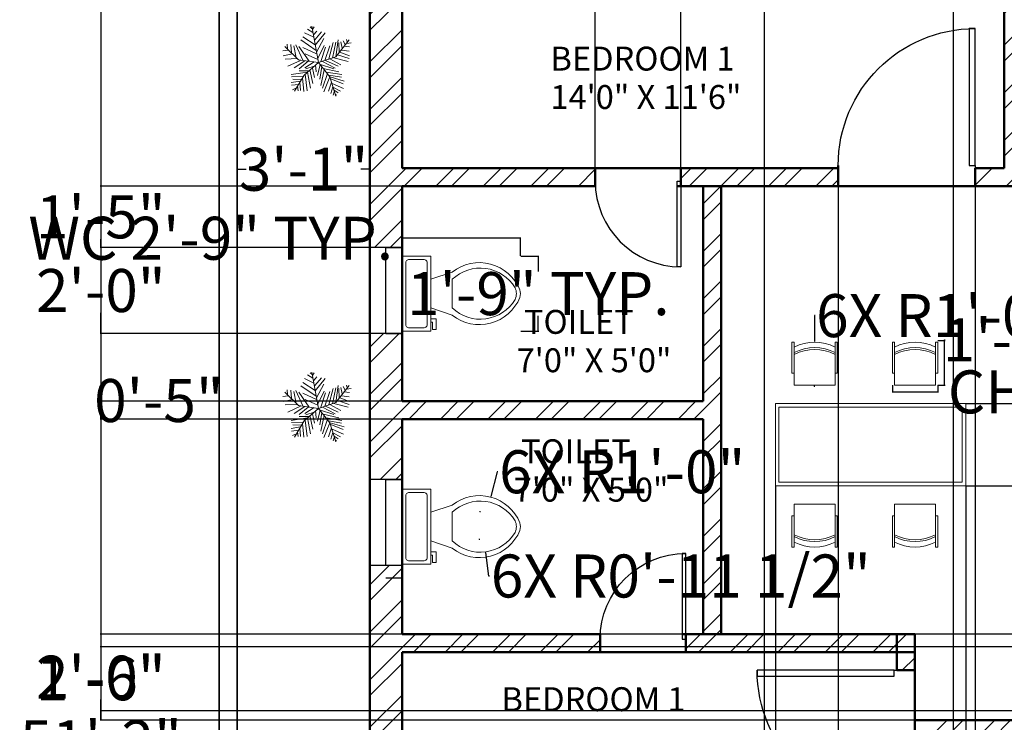
# Model space of a CAD drawing. Units: inches. Extents: x -40 to 578, y -482 to 237.
# Tile 4 of 7: x -26 to 249, y -129 to 67. Entities that reach past the tile are written whole.
import ezdxf

# ---------------------------------------------------------------- set-up
doc = ezdxf.new("R2010")
doc.units = ezdxf.units.IN
doc.header["$MEASUREMENT"] = 0
for name, color, linetype, lineweight in [('A-ANNO-DIMS', 2, 'Continuous', 18), ('A-AREA-IDEN', 240, 'Continuous', 25), ('A-FLOR-FIXT', 4, 'Continuous', 18), ('A-FURN', 4, 'Continuous', 18), ('A-WALL-PATT', 252, 'Continuous', 13), ('C-PROP', 3, 'Continuous', 35), ('DOORS', 2, 'Continuous', 25), ('L-PLNT', 94, 'Continuous', 13), ('WALLS', 3, 'Continuous', 50), ('WINDOWS', 241, 'Continuous', 25)]:
    doc.layers.add(name, color=color, linetype=linetype, lineweight=lineweight)
doc.styles.get("Standard").update_dxf_attribs({"font": 'arial.ttf'})
doc.dimstyles.get("Standard").update_dxf_attribs({"dimtxt": 12, "dimasz": 0.18, "dimexe": 0.18, "dimexo": 0.0625, "dimgap": 0.09, "dimtad": 0, "dimtih": 1, "dimtoh": 1, "dimdec": 0, "dimzin": 0, "dimdsep": 46, "dimlunit": 3, "dimtxsty": 'Standard', "dimcen": 0.09, "dimadec": 0, "dimazin": 0, "dimtfac": 1, "dimtdec": 0, "dimtofl": 0, "dimtmove": 0, "dimatfit": 3, "dimfxl": 1, "dimtolj": 1, "dimtzin": 0, "dimarcsym": 0})

# ---------------------------------------------------------------- blocks, each defined once
blk = doc.blocks.new('Toilet - top')
for p, q in [((9.5, -6), (9.5, -2)), ((-8, -8.5), (-8, -8)), ((-7, -8), (-7, -9.5)), ((-4, -8), (-6, -14)), ((4, -8), (6, -14)), ((-10, -8.5), (-8, -8.5)), ((-10, -9.5), (-10, -8.5)), ((-7, -9.5), (-10, -9.5)), ((4, -14), (-4, -14))]:
    blk.add_line(p, q)
blk.add_lwpolyline([(10.5, -8), (10.5, 0), (-10.5, 0), (-10.5, -8)], close=True)
for points in [[(-9.5, -2), (-9.5, -6)], [(8.5, -1), (-8.5, -1)], [(-8.5, -7), (8.5, -7)]]:
    blk.add_lwpolyline(points)
for centre, radius, start, end in [((-8.62, -1.88), 0.884, 81.8699, 188.1301), ((8.62, -1.88), 0.884, 351.8699, 98.1301), ((-8.62, -6.12), 0.884, 171.8699, 278.1301), ((8.62, -6.12), 0.884, 261.8699, 8.1301), ((3.52, -21.58), 12.17, 141.4691, 247.9714), ((4.2, -21.82), 11.33, 136.3677, 238.9468), ((-3.52, -21.58), 12.17, 292.0284, 38.5307), ((-4.2, -21.82), 11.33, 301.053, 43.6321), ((0, -27.88), 4, 245.7318, 294.2682), ((0, -29), 4, 254.8605, 285.1395)]:
    blk.add_arc(centre, radius, start, end)
blk = doc.blocks.new('*U10')
for p, q in [((0, 0), (0, -6)), ((40, 0), (40, -6))]:
    blk.add_line(p, q)
blk.add_lwpolyline([(0, 0), (0, 40), (1.75, 40), (1.75, 0)], close=True)
blk.add_arc((0, 0), 40, 0, 90)
blk = doc.blocks.new('*U14')
for p, q in [((-185.1152, 1008.5578), (-553.1612, 1185.4942)), ((-221.9198, 1197.3052), (-433.5526, 1338.8594)), ((-258.7244, 1362.456), (-332.3336, 1421.4348)), ((0, 0), (-266.7, 1447.8)), ((-231.1146, 1315.2628), (-166.7002, 1421.4348)), ((-194.31, 1102.9442), (-65.4812, 1256.284)), ((-148.3106, 914.1968), (118.5418, 1220.9018)), ((-129.8956, 701.8528), (265.7602, 1185.4942)), ((-93.091, 489.5342), (-700.3796, 902.3858)), ((-129.8956, 713.6638), (-626.7704, 1032.1544)), ((-74.7014, 418.7444), (219.7608, 961.39)), ((412.9786, 147.447), (587.8068, 796.2392)), ((560.197, 182.8292), (698.2206, 819.8358)), ((685.8, 228.6), (1219.2, 914.4)), ((689.0258, 230.0224), (790.2448, 914.1968)), ((891.4384, 831.6214), (946.658, 572.1096)), ((983.4626, 867.0036), (1066.2666, 725.4494)), ((1121.4862, 925.9824), (1149.0706, 831.6214)), ((-1206.4492, 501.3198), (-1418.082, 465.9376)), ((-800.1, 114.3), (-1333.5, 647.7)), ((-1234.059, 536.7274), (-1252.4486, 737.2604)), ((-1105.2302, 725.4494), (-1077.6458, 395.1732)), ((-976.4268, 666.4706), (-884.4026, 194.6402)), ((-902.8176, 713.6638), (-617.5756, 100.2538)), ((-369.1382, 53.086), (-783.1836, 642.874)), ((-617.5756, 607.4918), (-74.7014, 347.98)), ((-28.6766, 171.0436), (228.9556, 678.2816)), ((100.1268, 41.275), (284.1498, 619.2774)), ((256.5654, 88.4682), (449.7832, 666.4706)), ((808.6344, 784.4282), (827.0494, 418.7444)), ((845.439, 418.7444), (1241.0948, 277.1902)), ((919.0482, 501.3198), (1222.6798, 454.152)), ((1029.462, 654.685), (1241.0948, 631.0884)), ((1112.2914, 760.8316), (1296.3144, 784.4282)), ((-1031.621, 347.98), (-1399.667, 277.1902)), ((-847.598, 159.2326), (-1326.0578, 135.636)), ((-718.7946, 88.4682), (-1215.644, -147.447)), ((-543.9664, 76.6572), (-967.2066, -206.4512)), ((0, 0), (-800.1, 114.3)), ((-405.9428, 53.086), (-764.794, -241.8334)), ((0, 0), (-571.5, -495.3)), ((-166.7002, 29.4894), (-543.9664, -206.4512)), ((-525.5514, 347.98), (-28.6766, 123.8504)), ((0, 0), (685.8, 228.6)), ((0, 0), (457.2, -571.5)), ((164.5412, 41.275), (661.416, -218.2368)), ((284.1498, 88.4682), (781.0246, -147.447)), ((458.978, 147.447), (891.4384, -88.4682)), ((615.4166, 194.6402), (1185.8752, 41.275)), ((753.4148, 312.5978), (1222.6798, 159.2326)), ((-442.7474, -383.3876), (-1086.8406, -477.7486)), ((-387.5278, -324.4088), (-764.794, -324.4088)), ((-166.7002, -147.447), (-507.1618, -253.619)), ((-433.5526, -383.3876), (-323.1134, -1020.3688)), ((-341.5284, -289.0012), (-221.9198, -831.6214)), ((-240.3094, -218.2368), (-157.5054, -595.7062)), ((-120.7008, -88.4682), (-93.091, -371.5766)), ((63.3222, -76.6826), (-37.8714, -513.1308)), ((44.9326, -64.897), (615.4166, -241.8334)), ((127.7366, -159.258), (54.1274, -654.685)), ((228.9556, -289.0012), (90.932, -914.1968)), ((192.151, -230.0224), (817.8292, -371.5766)), ((311.7596, -383.3876), (937.4378, -477.7486)), ((-718.7946, -737.2604), (-1086.8406, -796.2392)), ((-617.5756, -548.5384), (-1077.6458, -560.324)), ((-681.9646, -666.496), (-1022.4262, -654.685)), ((-571.5, -495.3), (-952.5, -1143)), ((-737.1842, -784.4536), (-709.5744, -1114.7298)), ((-635.9652, -607.5172), (-580.771, -1150.1374)), ((-525.5514, -465.963), (-451.9422, -1126.5408)), ((357.759, -430.5554), (164.5412, -1020.3688)), ((458.978, -572.1096), (210.5406, -1161.923)), ((514.1976, -772.6426), (403.7838, -1138.3264)), ((412.9786, -501.3452), (919.0482, -583.9206)), ((457.2, -571.5), (685.8, -1333.5)), ((468.1982, -572.1096), (1029.462, -737.2604)), ((486.5878, -642.8994), (983.4626, -843.4324)), ((-783.1836, -867.029), (-1077.6458, -902.4112)), ((-875.2078, -1008.5832), (-1040.8412, -1079.3476)), ((-829.2084, -937.7934), (-810.7934, -1126.5408)), ((578.612, -961.39), (495.7826, -1232.7128)), ((541.8074, -831.6214), (992.6574, -1032.1544)), ((578.612, -973.1756), (873.0488, -1138.3264)), ((624.6114, -1161.923), (587.8068, -1291.6916)), ((624.6114, -1102.9442), (781.0246, -1209.1162)), ((679.8056, -1268.095), (716.6102, -1291.6916))]:
    blk.add_line(p, q)
blk = doc.blocks.new('*D20')
at = {"layer": 'A-ANNO-DIMS', "color": 0, "lineweight": -2, "transparency": 16777216}
for p, q in [((34.74, 26.4), (34.74, 24.97)), ((34.92, 25.15), (37.2, 25.15)), ((71.56, 25.15), (69.27, 25.15)), ((71.74, 26.4), (71.74, 24.97))]:
    blk.add_line(p, q, dxfattribs=at)
at = {"layer": 'A-ANNO-DIMS', "color": 0, "transparency": 16777216}
for points in [[(34.92, 25.18), (34.92, 25.12), (34.74, 25.15)], [(71.56, 25.18), (71.56, 25.12), (71.74, 25.15)]]:
    blk.add_solid(points, dxfattribs=at)
at = {"layer": 'Defpoints', "color": 0, "transparency": 16777216}
for p in [(34.74, 26.46), (34.74, 25.15), (71.74, 26.46)]:
    blk.add_point(p, dxfattribs=at)
at = {"layer": 'A-ANNO-DIMS', "color": 0, "transparency": 16777216, "insert": (53.24, 25.15), "char_height": 12, "attachment_point": 5}
blk.add_mtext('\\A1;3\'-1"', dxfattribs=at)
blk = doc.blocks.new('CHAIR-DINING')
for p, q in [((0.63, 0), (0.63, 10.59)), ((12.01, 10.59), (12.01, 0)), ((12.01, 0), (0.63, 0))]:
    blk.add_line(p, q)
for points in [[(0.63, 11.98), (0, 11.98), (0, 3.3), (0.63, 3.3)], [(12.64, 11.98), (12.01, 11.98), (12.01, 3.3), (12.64, 3.3)]]:
    blk.add_lwpolyline(points, close=True)
for centre in [(6.32, -0.34), (6.32, -1.87), (6.32, -2.38)]:
    blk.add_arc(centre, 12.32, 62.4906, 117.5094)
blk = doc.blocks.new('*D30')
at = {"layer": 'A-ANNO-DIMS', "color": 0, "lineweight": -2, "transparency": 16777216}
for p, q in [((217.52, -35.11), (217.52, -37.13)), ((230.16, -35.11), (230.16, -37.13)), ((217.7, -36.95), (229.98, -36.95)), ((230.16, -36.95), (230.34, -36.95))]:
    blk.add_line(p, q, dxfattribs=at)
at = {"layer": 'A-ANNO-DIMS', "color": 0, "transparency": 16777216}
for points in [[(217.7, -36.92), (217.7, -36.98), (217.52, -36.95)], [(229.98, -36.92), (229.98, -36.98), (230.16, -36.95)]]:
    blk.add_solid(points, dxfattribs=at)
at = {"layer": 'Defpoints', "color": 0, "transparency": 16777216}
for p in [(217.52, -35.05), (230.16, -35.05), (230.16, -36.95)]:
    blk.add_point(p, dxfattribs=at)
at = {"layer": 'A-ANNO-DIMS', "color": 0, "transparency": 16777216, "insert": (309.32, -36.95), "char_height": 12, "attachment_point": 5}
blk.add_mtext('\\A1;CHAIR 1\'-0 1/2" TYP.', dxfattribs=at)
blk = doc.blocks.new('*D31')
at = {"layer": 'A-ANNO-DIMS', "color": 0, "lineweight": -2, "transparency": 16777216}
for p, q in [((230.22, -22.61), (232.23, -22.61)), ((232.05, -22.61), (232.05, -22.43)), ((232.05, -22.43), (232.23, -22.43)), ((232.05, -34.87), (232.05, -22.79)), ((230.22, -35.05), (232.23, -35.05))]:
    blk.add_line(p, q, dxfattribs=at)
at = {"layer": 'A-ANNO-DIMS', "color": 0, "transparency": 16777216}
for points in [[(232.02, -22.79), (232.08, -22.79), (232.05, -22.61)], [(232.02, -34.87), (232.08, -34.87), (232.05, -35.05)]]:
    blk.add_solid(points, dxfattribs=at)
at = {"layer": 'Defpoints', "color": 0, "transparency": 16777216}
for p in [(230.16, -22.61), (232.05, -22.61), (230.16, -35.05)]:
    blk.add_point(p, dxfattribs=at)
at = {"layer": 'A-ANNO-DIMS', "color": 0, "transparency": 16777216, "insert": (282.31, -22.43), "char_height": 12, "attachment_point": 5}
blk.add_mtext('\\A1;1\'-0 1/2" TYP.', dxfattribs=at)
blk = doc.blocks.new('*D34')
at = {"layer": 'A-ANNO-DIMS', "color": 0, "lineweight": -2, "transparency": 16777216}
for p, q in [((80.74, 5.9), (80.56, 5.9)), ((80.74, 1.01), (80.74, 6.08)), ((113.6, 5.9), (80.92, 5.9)), ((113.78, 1.01), (113.78, 6.08))]:
    blk.add_line(p, q, dxfattribs=at)
at = {"layer": 'A-ANNO-DIMS', "color": 0, "transparency": 16777216}
for points in [[(80.92, 5.93), (80.92, 5.87), (80.74, 5.9)], [(113.6, 5.93), (113.6, 5.87), (113.78, 5.9)]]:
    blk.add_solid(points, dxfattribs=at)
at = {"layer": 'Defpoints', "color": 0, "transparency": 16777216}
for p in [(80.74, 5.9), (80.74, 0.95), (113.78, 0.95)]:
    blk.add_point(p, dxfattribs=at)
at = {"layer": 'A-ANNO-DIMS', "color": 0, "transparency": 16777216, "insert": (27.36, 5.9), "char_height": 12, "attachment_point": 5}
blk.add_mtext('\\A1;WC 2\'-9" TYP.', dxfattribs=at)
blk = doc.blocks.new('*D35')
at = {"layer": 'A-ANNO-DIMS', "color": 0, "lineweight": -2, "transparency": 16777216}
for p, q in [((113.85, 0.95), (118.92, 0.95)), ((118.74, 0.77), (118.74, -3.34)), ((118.74, -19.87), (118.74, -15.77)), ((113.85, -20.05), (118.92, -20.05))]:
    blk.add_line(p, q, dxfattribs=at)
at = {"layer": 'A-ANNO-DIMS', "color": 0, "transparency": 16777216}
for points in [[(118.71, 0.77), (118.77, 0.77), (118.74, 0.95)], [(118.71, -19.87), (118.77, -19.87), (118.74, -20.05)]]:
    blk.add_solid(points, dxfattribs=at)
at = {"layer": 'Defpoints', "color": 0, "transparency": 16777216}
for p in [(113.78, 0.95), (118.74, 0.95), (113.78, -20.05)]:
    blk.add_point(p, dxfattribs=at)
at = {"layer": 'A-ANNO-DIMS', "color": 0, "transparency": 16777216, "insert": (118.74, -9.55), "char_height": 12, "attachment_point": 5}
blk.add_mtext('\\A1;1\'-9" TYP.', dxfattribs=at)
blk = doc.blocks.new('*D42')
at = {"layer": 'A-ANNO-DIMS', "color": 0, "lineweight": -2, "transparency": 16777216}
for p, q in [((71.78, -441.49), (71.78, 219.12)), ((71.96, 218.94), (110.77, 218.94)), ((181.65, 218.94), (142.84, 218.94)), ((181.83, -441.49), (181.83, 219.12))]:
    blk.add_line(p, q, dxfattribs=at)
at = {"layer": 'A-ANNO-DIMS', "color": 0, "transparency": 16777216}
for points in [[(71.96, 218.97), (71.96, 218.91), (71.78, 218.94)], [(181.65, 218.97), (181.65, 218.91), (181.83, 218.94)]]:
    blk.add_solid(points, dxfattribs=at)
at = {"layer": 'Defpoints', "color": 0, "transparency": 16777216}
for p in [(181.83, 218.94), (71.78, -441.55), (181.83, -441.55)]:
    blk.add_point(p, dxfattribs=at)
at = {"layer": 'A-ANNO-DIMS', "color": 0, "transparency": 16777216, "insert": (126.81, 218.94), "char_height": 12, "attachment_point": 5}
blk.add_mtext('\\A1;9\'-2"', dxfattribs=at)
blk = doc.blocks.new('*D44')
at = {"layer": 'A-ANNO-DIMS', "color": 0, "lineweight": -2, "transparency": 16777216}
for p, q in [((29.68, 172.45), (-3.49, 172.45)), ((-3.31, 172.27), (-3.31, -128.34)), ((-3.31, -441.37), (-3.31, -140.77)), ((29.68, -441.55), (-3.49, -441.55))]:
    blk.add_line(p, q, dxfattribs=at)
at = {"layer": 'A-ANNO-DIMS', "color": 0, "transparency": 16777216}
for points in [[(-3.34, 172.27), (-3.28, 172.27), (-3.31, 172.45)], [(-3.34, -441.37), (-3.28, -441.37), (-3.31, -441.55)]]:
    blk.add_solid(points, dxfattribs=at)
at = {"layer": 'Defpoints', "color": 0, "transparency": 16777216}
for p in [(-3.31, 172.45), (29.74, 172.45), (29.74, -441.55)]:
    blk.add_point(p, dxfattribs=at)
at = {"layer": 'A-ANNO-DIMS', "color": 0, "transparency": 16777216, "insert": (-3.31, -134.55), "char_height": 12, "attachment_point": 5}
blk.add_mtext('\\A1;51\'-2"', dxfattribs=at)
blk = doc.blocks.new('*D52')
at = {"layer": 'A-ANNO-DIMS', "color": 0, "lineweight": -2, "transparency": 16777216}
for p, q in [((234.57, -377.49), (234.57, 219.12)), ((234.75, 218.94), (265.48, 218.94)), ((265.66, -377.49), (265.66, 219.12)), ((265.66, 218.94), (265.84, 218.94))]:
    blk.add_line(p, q, dxfattribs=at)
at = {"layer": 'A-ANNO-DIMS', "color": 0, "transparency": 16777216}
for points in [[(234.75, 218.97), (234.75, 218.91), (234.57, 218.94)], [(265.48, 218.97), (265.48, 218.91), (265.66, 218.94)]]:
    blk.add_solid(points, dxfattribs=at)
at = {"layer": 'Defpoints', "color": 0, "transparency": 16777216}
for p in [(265.66, 218.94), (234.57, -377.55), (265.66, -377.55)]:
    blk.add_point(p, dxfattribs=at)
at = {"layer": 'A-ANNO-DIMS', "color": 0, "transparency": 16777216, "insert": (281.98, 218.94), "char_height": 12, "attachment_point": 5}
blk.add_mtext('\\A1;2\'-7"', dxfattribs=at)
blk = doc.blocks.new('*D54')
at = {"layer": 'A-ANNO-DIMS', "color": 0, "lineweight": -2, "transparency": 16777216}
for p, q in [((202.4, 25.39), (202.4, -474.78)), ((240.62, 25.39), (240.62, -474.78)), ((202.58, -474.6), (205.48, -474.6)), ((240.44, -474.6), (237.55, -474.6))]:
    blk.add_line(p, q, dxfattribs=at)
at = {"layer": 'A-ANNO-DIMS', "color": 0, "transparency": 16777216}
for points in [[(202.58, -474.57), (202.58, -474.63), (202.4, -474.6)], [(240.44, -474.57), (240.44, -474.63), (240.62, -474.6)]]:
    blk.add_solid(points, dxfattribs=at)
at = {"layer": 'Defpoints', "color": 0, "transparency": 16777216}
for p in [(202.4, 25.45), (240.62, 25.45), (240.62, -474.6)]:
    blk.add_point(p, dxfattribs=at)
at = {"layer": 'A-ANNO-DIMS', "color": 0, "transparency": 16777216, "insert": (221.51, -474.6), "char_height": 12, "attachment_point": 5}
blk.add_mtext('\\A1;3\'-2"', dxfattribs=at)
blk = doc.blocks.new('*D55')
at = {"layer": 'A-ANNO-DIMS', "color": 0, "lineweight": -2, "transparency": 16777216}
for p, q in [((134.6, 25.51), (134.6, 219.12)), ((134.78, 218.94), (158.35, 218.94)), ((158.53, 25.51), (158.53, 219.12)), ((158.53, 218.94), (158.71, 218.94))]:
    blk.add_line(p, q, dxfattribs=at)
at = {"layer": 'A-ANNO-DIMS', "color": 0, "transparency": 16777216}
for points in [[(134.78, 218.97), (134.78, 218.91), (134.6, 218.94)], [(158.35, 218.97), (158.35, 218.91), (158.53, 218.94)]]:
    blk.add_solid(points, dxfattribs=at)
at = {"layer": 'Defpoints', "color": 0, "transparency": 16777216}
for p in [(158.53, 218.94), (134.6, 25.45), (158.53, 25.45)]:
    blk.add_point(p, dxfattribs=at)
at = {"layer": 'A-ANNO-DIMS', "color": 0, "transparency": 16777216, "insert": (174.86, 218.94), "char_height": 12, "attachment_point": 5}
blk.add_mtext('\\A1;2\'-0"', dxfattribs=at)
blk = doc.blocks.new('*D56')
at = {"layer": 'A-ANNO-DIMS', "color": 0, "lineweight": -2, "transparency": 16777216}
for p, q in [((71.68, 3.32), (-3.49, 3.32)), ((-3.31, 3.14), (-3.31, -2.46)), ((-3.31, -20.5), (-3.31, -14.9)), ((71.68, -20.68), (-3.49, -20.68))]:
    blk.add_line(p, q, dxfattribs=at)
at = {"layer": 'A-ANNO-DIMS', "color": 0, "transparency": 16777216}
for points in [[(-3.34, 3.14), (-3.28, 3.14), (-3.31, 3.32)], [(-3.34, -20.5), (-3.28, -20.5), (-3.31, -20.68)]]:
    blk.add_solid(points, dxfattribs=at)
at = {"layer": 'Defpoints', "color": 0, "transparency": 16777216}
for p in [(-3.31, 3.32), (71.74, 3.32), (71.74, -20.68)]:
    blk.add_point(p, dxfattribs=at)
at = {"layer": 'A-ANNO-DIMS', "color": 0, "transparency": 16777216, "insert": (-3.31, -8.68), "char_height": 12, "attachment_point": 5}
blk.add_mtext('\\A1;2\'-0"', dxfattribs=at)
blk = doc.blocks.new('*D57')
at = {"layer": 'A-ANNO-DIMS', "color": 0, "lineweight": -2, "transparency": 16777216}
for p, q in [((164.68, -39.55), (-3.49, -39.55)), ((-3.31, -39.55), (-3.31, -39.37)), ((-3.31, -39.37), (-3.13, -39.37)), ((-3.31, -44.37), (-3.31, -39.73)), ((164.68, -44.55), (-3.49, -44.55))]:
    blk.add_line(p, q, dxfattribs=at)
at = {"layer": 'A-ANNO-DIMS', "color": 0, "transparency": 16777216}
for points in [[(-3.34, -39.73), (-3.28, -39.73), (-3.31, -39.55)], [(-3.34, -44.37), (-3.28, -44.37), (-3.31, -44.55)]]:
    blk.add_solid(points, dxfattribs=at)
at = {"layer": 'Defpoints', "color": 0, "transparency": 16777216}
for p in [(-3.31, -39.55), (164.74, -39.55), (164.74, -44.55)]:
    blk.add_point(p, dxfattribs=at)
at = {"layer": 'A-ANNO-DIMS', "color": 0, "transparency": 16777216, "insert": (12.91, -39.37), "char_height": 12, "attachment_point": 5}
blk.add_mtext('\\A1;0\'-5"', dxfattribs=at)
blk = doc.blocks.new('*D58')
at = {"layer": 'A-ANNO-DIMS', "color": 0, "lineweight": -2, "transparency": 16777216}
for p, q in [((80.68, 20.45), (-3.49, 20.45)), ((-3.31, 20.27), (-3.31, 18.1)), ((-3.31, 3.5), (-3.31, 5.67)), ((80.68, 3.32), (-3.49, 3.32))]:
    blk.add_line(p, q, dxfattribs=at)
at = {"layer": 'A-ANNO-DIMS', "color": 0, "transparency": 16777216}
for points in [[(-3.34, 20.27), (-3.28, 20.27), (-3.31, 20.45)], [(-3.34, 3.5), (-3.28, 3.5), (-3.31, 3.32)]]:
    blk.add_solid(points, dxfattribs=at)
at = {"layer": 'Defpoints', "color": 0, "transparency": 16777216}
for p in [(-3.31, 20.45), (80.74, 20.45), (80.74, 3.32)]:
    blk.add_point(p, dxfattribs=at)
at = {"layer": 'A-ANNO-DIMS', "color": 0, "transparency": 16777216, "insert": (-3.31, 11.88), "char_height": 12, "attachment_point": 5}
blk.add_mtext('\\A1;1\'-5"', dxfattribs=at)
blk = doc.blocks.new('*D66')
at = {"layer": 'A-ANNO-DIMS', "color": 0, "lineweight": -2, "transparency": 16777216}
for p, q in [((289.5, -104.55), (-3.49, -104.55)), ((-3.31, -104.73), (-3.31, -110.34)), ((-3.31, -128.37), (-3.31, -122.77)), ((289.5, -128.55), (-3.49, -128.55))]:
    blk.add_line(p, q, dxfattribs=at)
at = {"layer": 'A-ANNO-DIMS', "color": 0, "transparency": 16777216}
for points in [[(-3.34, -104.73), (-3.28, -104.73), (-3.31, -104.55)], [(-3.34, -128.37), (-3.28, -128.37), (-3.31, -128.55)]]:
    blk.add_solid(points, dxfattribs=at)
at = {"layer": 'Defpoints', "color": 0, "transparency": 16777216}
for p in [(289.56, -104.55), (-3.31, -128.55), (289.56, -128.55)]:
    blk.add_point(p, dxfattribs=at)
at = {"layer": 'A-ANNO-DIMS', "color": 0, "transparency": 16777216, "insert": (-3.31, -116.55), "char_height": 12, "attachment_point": 5}
blk.add_mtext('\\A1;2\'-0"', dxfattribs=at)
blk = doc.blocks.new('*D68')
at = {"layer": 'A-ANNO-DIMS', "color": 0, "lineweight": -2, "transparency": 16777216}
for p, q in [((321.44, -108.06), (-3.49, -108.06)), ((-3.31, -108.24), (-3.31, -110.78)), ((-3.31, -125.74), (-3.31, -123.21)), ((321.44, -125.92), (-3.49, -125.92))]:
    blk.add_line(p, q, dxfattribs=at)
at = {"layer": 'A-ANNO-DIMS', "color": 0, "transparency": 16777216}
for points in [[(-3.34, -108.24), (-3.28, -108.24), (-3.31, -108.06)], [(-3.34, -125.74), (-3.28, -125.74), (-3.31, -125.92)]]:
    blk.add_solid(points, dxfattribs=at)
at = {"layer": 'Defpoints', "color": 0, "transparency": 16777216}
for p in [(321.5, -108.06), (-3.31, -125.92), (321.5, -125.92)]:
    blk.add_point(p, dxfattribs=at)
at = {"layer": 'A-ANNO-DIMS', "color": 0, "transparency": 16777216, "insert": (-3.31, -116.99), "char_height": 12, "attachment_point": 5}
blk.add_mtext('\\A1;1\'-6"', dxfattribs=at)
blk = doc.blocks.new('*D71')
at = {"layer": 'A-ANNO-DIMS', "color": 0, "lineweight": -2, "transparency": 16777216}
for p, q in [((184.88, -63.19), (184.88, -474.78)), ((237.97, -63.19), (237.97, -474.78)), ((185.06, -474.6), (195.15, -474.6)), ((237.79, -474.6), (227.71, -474.6))]:
    blk.add_line(p, q, dxfattribs=at)
at = {"layer": 'A-ANNO-DIMS', "color": 0, "transparency": 16777216}
for points in [[(185.06, -474.57), (185.06, -474.63), (184.88, -474.6)], [(237.79, -474.57), (237.79, -474.63), (237.97, -474.6)]]:
    blk.add_solid(points, dxfattribs=at)
at = {"layer": 'Defpoints', "color": 0, "transparency": 16777216}
for p in [(184.88, -63.12), (237.97, -63.12), (237.97, -474.6)]:
    blk.add_point(p, dxfattribs=at)
at = {"layer": 'A-ANNO-DIMS', "color": 0, "transparency": 16777216, "insert": (211.43, -474.6), "char_height": 12, "attachment_point": 5}
blk.add_mtext('\\A1;4\'-5"', dxfattribs=at)
blk = doc.blocks.new('*D72')
at = {"layer": 'A-ANNO-DIMS', "color": 0, "lineweight": -2, "transparency": 16777216}
for p, q in [((238.04, -40.21), (516.97, -40.21)), ((516.79, -40.39), (516.79, -45.55)), ((516.79, -62.94), (516.79, -57.78)), ((238.04, -63.12), (516.97, -63.12))]:
    blk.add_line(p, q, dxfattribs=at)
at = {"layer": 'A-ANNO-DIMS', "color": 0, "transparency": 16777216}
for points in [[(516.76, -40.39), (516.82, -40.39), (516.79, -40.21)], [(516.76, -62.94), (516.82, -62.94), (516.79, -63.12)]]:
    blk.add_solid(points, dxfattribs=at)
at = {"layer": 'Defpoints', "color": 0, "transparency": 16777216}
for p in [(237.97, -40.21), (516.79, -40.21), (237.97, -63.12)]:
    blk.add_point(p, dxfattribs=at)
at = {"layer": 'A-ANNO-DIMS', "color": 0, "transparency": 16777216, "insert": (516.79, -51.67), "char_height": 12, "attachment_point": 5}
blk.add_mtext('\\A1;1\'-11"', dxfattribs=at)
blk = doc.blocks.new('*D82')
at = {"layer": 'A-ANNO-DIMS', "color": 0, "lineweight": -2, "transparency": 16777216}
for p, q in [((196.01, -15.68), (195.83, -15.68)), ((195.83, -15.68), (195.83, -22.89)), ((195.74, -35.39), (195.92, -35.39)), ((195.83, -35.48), (195.83, -35.3))]:
    blk.add_line(p, q, dxfattribs=at)
at = {"layer": 'A-ANNO-DIMS', "color": 0, "transparency": 16777216}
blk.add_solid([(195.8, -22.89), (195.86, -22.89), (195.83, -23.07)], dxfattribs=at)
at = {"layer": 'Defpoints', "color": 0, "transparency": 16777216}
for p in [(195.83, -23.07), (195.83, -35.39)]:
    blk.add_point(p, dxfattribs=at)
at = {"layer": 'A-ANNO-DIMS', "color": 0, "transparency": 16777216, "insert": (244.7, -15.68), "char_height": 12, "attachment_point": 5}
blk.add_mtext('\\A1;6X R1\'-0 1/2"', dxfattribs=at)
blk = doc.blocks.new('*D83')
at = {"layer": 'A-ANNO-DIMS', "color": 0, "lineweight": -2, "transparency": 16777216}
for p, q in [((107.27, -59.24), (105.46, -66.13)), ((107.45, -59.24), (107.27, -59.24)), ((102.23, -78.07), (102.41, -78.07)), ((102.32, -78.16), (102.32, -77.98))]:
    blk.add_line(p, q, dxfattribs=at)
at = {"layer": 'A-ANNO-DIMS', "color": 0, "transparency": 16777216}
blk.add_solid([(105.43, -66.12), (105.48, -66.14), (105.41, -66.3)], dxfattribs=at)
at = {"layer": 'Defpoints', "color": 0, "transparency": 16777216}
for p in [(105.41, -66.3), (102.32, -78.07)]:
    blk.add_point(p, dxfattribs=at)
at = {"layer": 'A-ANNO-DIMS', "color": 0, "transparency": 16777216, "insert": (142.15, -59.24), "char_height": 12, "attachment_point": 5}
blk.add_mtext('\\A1;6X R1\'-0"', dxfattribs=at)
blk = doc.blocks.new('*D84')
at = {"layer": 'A-ANNO-DIMS', "color": 0, "lineweight": -2, "transparency": 16777216}
for p, q in [((102.47, -70.35), (102.65, -70.35)), ((102.56, -70.44), (102.56, -70.26)), ((104.97, -88.32), (104.09, -81.76)), ((105.15, -88.32), (104.97, -88.32))]:
    blk.add_line(p, q, dxfattribs=at)
at = {"layer": 'A-ANNO-DIMS', "color": 0, "transparency": 16777216}
blk.add_solid([(104.12, -81.76), (104.06, -81.76), (104.06, -81.58)], dxfattribs=at)
at = {"layer": 'Defpoints', "color": 0, "transparency": 16777216}
for p in [(102.56, -70.35), (104.06, -81.58)]:
    blk.add_point(p, dxfattribs=at)
at = {"layer": 'A-ANNO-DIMS', "color": 0, "transparency": 16777216, "insert": (158.5, -88.32), "char_height": 12, "attachment_point": 5}
blk.add_mtext('\\A1;6X R0\'-11 1/2"', dxfattribs=at)

msp = doc.modelspace()

# ---------------------------------------------------------------- hatches: boundary and pattern name
at = {"layer": 'A-WALL-PATT'}
h = msp.add_hatch(dxfattribs=at)
h.set_pattern_fill('ANSI32', color=256, scale=25)
h.set_pattern_definition([(45, (-1993.713, -1175.095), (-6.629126, 6.629126), []), (45, (-1989.294, -1175.095), (-6.629126, 6.629126), [])])
h.paths.add_polyline_path([(248.74, 172.45), (71.74, 172.45), (71.74, 114.63), (80.74, 114.63), (80.74, 163.45), (248.74, 163.45)])
h.paths.add_polyline_path([(253.74, 172.45), (248.74, 172.45), (248.74, 163.45), (253.74, 163.45)])
h.paths.add_polyline_path([(253.74, 163.45), (248.74, 163.45), (248.74, 25.45), (240.62, 25.45), (240.62, 20.45), (263.71, 20.45), (263.71, 25.45), (253.74, 25.45)])
h.paths.add_polyline_path([(483.74, 172.45), (253.74, 172.45), (253.74, 163.45), (426.74, 163.45), (474.74, 163.45), (474.74, 79.45), (465.23, 79.45), (465.23, 77.2), (441.23, 77.2), (441.23, 74.45), (483.74, 74.45)])
h.paths.add_polyline_path([(80.74, 78.63), (71.74, 78.63), (71.74, 3.32), (80.74, 3.32), (80.74, 20.45), (134.6, 20.45), (134.6, 25.45), (80.74, 25.45)])
h.paths.add_polyline_path([(202.4, 25.45), (158.53, 25.45), (158.53, 20.45), (202.4, 20.45)])
h.paths.add_polyline_path([(169.74, 20.45), (164.74, 20.45), (164.74, -39.55), (80.74, -39.55), (80.74, -20.68), (71.74, -20.68), (71.74, -61.38), (80.74, -61.38), (80.74, -44.55), (164.74, -44.55), (164.74, -104.55), (169.74, -104.55), (169.74, -44.55)])
h.paths.add_polyline_path([(135.96, -104.55), (80.74, -104.55), (80.74, -85.38), (71.74, -85.38), (71.74, -155.89), (80.74, -155.89), (80.74, -109.55), (135.96, -109.55)])
h.paths.add_polyline_path([(218.74, -104.55), (159.9, -104.55), (159.9, -109.55), (218.74, -109.55)])
h.paths.add_polyline_path([(223.74, -104.55), (218.74, -104.55), (218.74, -109.55), (223.74, -109.55)])
h.paths.add_polyline_path([(223.74, -109.55), (218.74, -109.55), (218.74, -114.58), (223.74, -114.58)])
h.paths.add_polyline_path([(430.74, -85.66), (421.74, -85.66), (421.74, -128.55), (223.74, -128.55), (223.74, -133.55), (421.74, -133.55), (421.74, -197.77), (430.74, -197.77)])
h.paths.add_polyline_path([(223.74, -152.8), (218.74, -152.8), (218.74, -229.55), (151.59, -229.55), (151.59, -238.55), (223.74, -238.55), (223.74, -229.55)])
h.paths.add_polyline_path([(115.59, -229.55), (98.23, -229.55), (80.74, -229.55), (80.74, -212.75), (80.74, -191.89), (71.74, -191.89), (71.74, -238.55), (115.59, -238.55)])
h.paths.add_polyline_path([(307.53, -289.55), (223.74, -289.55), (223.74, -283.47), (218.74, -283.47), (218.74, -298.55), (307.53, -298.55)])
h.paths.add_polyline_path([(421.74, -289.55), (343.53, -289.55), (343.53, -298.55), (421.74, -298.55)])
h.paths.add_polyline_path([(430.74, -367.34), (421.74, -367.34), (421.74, -377.55), (234.57, -377.55), (234.57, -386.55), (430.74, -386.55)])
h.paths.add_polyline_path([(430.74, -298.55), (430.74, -233.77), (421.74, -233.77), (421.74, -289.55), (421.74, -298.55), (421.74, -331.34), (430.74, -331.34)])
h.paths.add_polyline_path([(430.74, -11.67), (427.15, -11.67, -0.057068), (421.74, -11.05), (421.74, -49.66), (430.74, -49.66)])
h.paths.add_polyline_path([(430.74, 31.9), (421.74, 31.9), (421.74, 25.45), (301.93, 25.45), (301.93, 20.45), (421.74, 20.45), (421.74, 12.26), (430.74, 12.26)])
h.paths.add_polyline_path([(426.74, 134.23, -0.014739), (425.33, 134.19), (421.74, 134.19), (421.74, 74.45), (441.23, 74.45), (441.23, 77.2), (441.23, 79.45), (426.74, 79.45)], flags=17)
h.paths.add_polyline_path([(430.74, 74.45), (421.74, 74.45), (421.74, 67.9), (430.74, 67.9)])

# ---------------------------------------------------------------- linework, layer by layer
at = {"layer": 'A-FURN'}
for points in [[(237.97, -63.12), (184.88, -63.12), (184.88, -40.21), (237.97, -40.21)], [(236.97, -62.12), (185.88, -62.12), (185.88, -41.21), (236.97, -41.21)]]:
    msp.add_lwpolyline(points, close=True, dxfattribs=at)
at = {"layer": 'C-PROP'}
for p, q in [((29.74, 172.45), (29.74, -441.55)), ((34.74, 167.45), (34.74, -432.55))]:
    msp.add_line(p, q, dxfattribs=at)
at = {"layer": 'WALLS'}
for p, q in [((71.74, 172.45), (71.74, -238.55)), ((248.74, 172.45), (248.74, 25.45)), ((80.74, 163.45), (80.74, 25.45)), ((202.4, 25.45), (80.74, 25.45)), ((134.6, 25.45), (134.6, 20.45)), ((158.53, 25.45), (158.53, 20.45)), ((202.4, 20.45), (202.4, 26.18)), ((240.62, 25.45), (240.62, 20.45)), ((248.74, 25.45), (240.62, 25.45)), ((80.74, 20.45), (80.74, -39.55)), ((134.64, 20.45), (80.74, 20.45)), ((421.74, 20.45), (157.49, 20.45)), ((164.74, 20.45), (164.74, -39.55)), ((169.74, 20.45), (169.74, -44.55)), ((164.74, -39.55), (80.74, -39.55)), ((80.74, -44.55), (80.74, -104.55)), ((164.74, -44.55), (80.74, -44.55)), ((164.74, -44.55), (164.74, -104.55)), ((169.74, -44.55), (169.74, -104.55)), ((136.01, -104.55), (80.74, -104.55)), ((135.96, -104.55), (135.96, -109.55)), ((223.74, -104.55), (158.85, -104.55)), ((159.9, -104.55), (159.9, -109.55)), ((218.74, -104.55), (218.74, -114.58)), ((223.74, -104.55), (223.74, -229.55)), ((80.74, -109.55), (80.74, -229.55)), ((223.74, -109.55), (80.74, -109.55)), ((223.74, -114.58), (218.74, -114.58)), ((223.74, -128.55), (421.74, -128.55))]:
    msp.add_line(p, q, dxfattribs=at)
at = {"layer": 'WINDOWS'}
for p, q in [((80.74, 3.32), (71.74, 3.32)), ((76.24, -20.68), (76.24, 3.32)), ((76.24, 3.32), (80.74, 3.32)), ((80.74, -20.68), (71.74, -20.68)), ((76.24, -20.68), (80.74, -20.68)), ((80.74, -61.38), (71.74, -61.38)), ((76.24, -85.38), (76.24, -61.38)), ((76.24, -61.38), (80.74, -61.38)), ((80.74, -85.38), (71.74, -85.38)), ((76.24, -88.85), (80.74, -88.85))]:
    msp.add_line(p, q, dxfattribs=at)

# ---------------------------------------------------------------- block references
at = {"layer": 'A-FLOR-FIXT', "rotation": 90}
for p in [(80.74, -9.55), (80.74, -74.55)]:
    msp.add_blockref('Toilet - top', p, dxfattribs=at)
at = {"layer": 'A-FURN'}
for p in [(189.51, -35.05), (217.52, -35.05)]:
    msp.add_blockref('CHAIR-DINING', p, dxfattribs=at)
at = {"layer": 'A-FURN', "extrusion": (0, 0, -1), "zscale": -1, "rotation": 180}
for p in [(-189.51, -68.28), (-217.52, -68.28)]:
    msp.add_blockref('CHAIR-DINING', p, dxfattribs=at)
at = {"layer": 'DOORS'}
for p, xscale, yscale, zscale in [((240.62, 26.18), -0.9555568703817776, 0.9555568703817776, 0.9555568703817776), ((159.9, -105.96), -0.5983195859330738, 0.5983195859330738, 0.5983195859330738)]:
    msp.add_blockref('*U10', p, dxfattribs=dict(at, xscale=xscale, yscale=yscale, zscale=zscale))
for p, xscale, yscale, zscale, rotation in [((158.53, 21.86), 0.5983195859330738, 0.5983195859330738, 0.5983195859330738, 180), ((218, -114.58), -0.9555568703817776, 0.9555568703817776, 0.9555568703817776, 90)]:
    msp.add_blockref('*U10', p, dxfattribs=dict(at, xscale=xscale, yscale=yscale, zscale=zscale, rotation=rotation))
at = {"layer": 'L-PLNT', "xscale": 0.0070029080995801, "yscale": 0.0070029080995801, "zscale": 0.0070029080995801}
for p in [(57.41, 54.9), (57.41, -41.55)]:
    msp.add_blockref('*U14', p, dxfattribs=at)

# ---------------------------------------------------------------- texts
at = {"layer": 'A-AREA-IDEN'}
for s, height, p in [('BEDROOM 1', 6.67, (122.13, 52.68)), ('14\'0" X 11\'6"', 6.6698, (122.13, 41.97)), ('   TOILET', 6.67, (108.62, -20.76)), ('  7\'0" X 5\'0"', 6.6698, (108.62, -31.47)), ('   TOILET', 6.67, (107.8, -56.86)), ('  7\'0" X 5\'0"', 6.6698, (107.8, -67.57)), ('BEDROOM 1', 6.67, (108.47, -126.02))]:
    msp.add_text(s, height=height, dxfattribs=at).set_placement(p)

# ---------------------------------------------------------------- dimensions: what is measured, and where the dimension line sits
at = {"layer": 'A-ANNO-DIMS'}
for base, p1, p2, override, picture, middle in [((181.8272, 218.9381), (71.7835, -441.5525), (181.8272, -441.5525), {"dimdec": 1, "dimlfac": 1, "dimrnd": 0, "dimzin": 1, "dimdsep": 46, "dimlunit": 4, "dimfrac": 2}, '*D42', (126.8054, 218.9381)), ((158.53, 218.94), (134.6, 25.45), (158.53, 25.45), {"dimdec": 1, "dimlfac": 1, "dimrnd": 0, "dimzin": 1, "dimdsep": 46, "dimlunit": 4, "dimfrac": 2}, '*D55', (174.86, 218.94)), ((265.66, 218.94), (234.57, -377.55), (265.66, -377.55), {"dimdec": 1, "dimlfac": 1, "dimrnd": 0, "dimzin": 1, "dimdsep": 46, "dimlunit": 4, "dimfrac": 2}, '*D52', (281.98, 218.94)), ((34.74, 25.15), (71.74, 26.46), (34.74, 26.46), {"dimclrd": 0, "dimclre": 0, "dimclrt": 0}, '*D20', (53.24, 25.15)), ((240.62, -474.6), (202.4, 25.45), (240.62, 25.45), {"dimdec": 1, "dimlfac": 1, "dimrnd": 0, "dimzin": 1, "dimdsep": 46, "dimlunit": 4, "dimfrac": 2}, '*D54', (221.51, -474.6)), ((237.97, -474.6), (184.88, -63.12), (237.97, -63.12), {"dimdec": 1, "dimlfac": 1, "dimrnd": 0, "dimzin": 1, "dimdsep": 46, "dimlunit": 4, "dimfrac": 2}, '*D71', (211.43, -474.6))]:
    dim = msp.add_linear_dim(base=base, p1=p1, p2=p2, dimstyle='Standard', override=override, dxfattribs=at)
    dim.commit()
    dim.dimension.update_dxf_attribs({"geometry": picture, "text_midpoint": middle})
for base, p1, p2, picture, middle in [((-3.31, 172.45), (29.74, -441.55), (29.74, 172.45), '*D44', (-3.31, -134.55)), ((-3.31, 20.45), (80.74, 3.32), (80.74, 20.45), '*D58', (-3.31, 11.88)), ((-3.31, 3.32), (71.74, -20.68), (71.74, 3.32), '*D56', (-3.31, -8.68)), ((-3.31, -39.55), (164.74, -44.55), (164.74, -39.55), '*D57', (12.91, -39.37)), ((516.79, -40.21), (237.97, -63.12), (237.97, -40.21), '*D72', (516.79, -51.67)), ((-3.31, -128.55), (289.56, -104.55), (289.56, -128.55), '*D66', (-3.31, -116.55)), ((-3.31, -125.92), (321.5, -108.06), (321.5, -125.92), '*D68', (-3.31, -116.99))]:
    dim = msp.add_linear_dim(base=base, p1=p1, p2=p2, angle=90, dimstyle='Standard', override={"dimdec": 1, "dimlfac": 1, "dimrnd": 0, "dimzin": 1, "dimdsep": 46, "dimlunit": 4, "dimfrac": 2}, dxfattribs=at)
    dim.commit()
    dim.dimension.update_dxf_attribs({"geometry": picture, "text_midpoint": middle})
for base, p1, p2, angle, text, picture, middle in [((80.74, 5.9), (113.78, 0.95), (80.74, 0.95), 180, 'WC <> TYP.', '*D34', (27.36, 5.9)), ((118.74, 0.95), (113.78, -20.05), (113.78, 0.95), 90, '<> TYP.', '*D35', (118.74, -9.55)), ((232.05, -22.61), (230.16, -35.05), (230.16, -22.61), 90, '<> TYP.', '*D31', (282.31, -22.43))]:
    dim = msp.add_linear_dim(base=base, p1=p1, p2=p2, angle=angle, text=text, dimstyle='Standard', override={"dimdec": 1, "dimlfac": 1, "dimrnd": 0, "dimzin": 1, "dimdsep": 46, "dimlunit": 4, "dimfrac": 2}, dxfattribs=at)
    dim.commit()
    dim.dimension.update_dxf_attribs({"geometry": picture, "text_midpoint": middle})
for center, mpoint, picture, middle in [((195.83, -35.39), (195.83, -23.07), '*D82', (244.7, -15.68)), ((102.32, -78.07), (105.41, -66.3), '*D83', (142.15, -59.24)), ((102.56, -70.35), (104.06, -81.58), '*D84', (158.5, -88.32))]:
    dim = msp.add_radius_dim(center=center, mpoint=mpoint, text='6X <>', dimstyle='Standard', override={"dimdec": 1, "dimlfac": 1, "dimrnd": 0, "dimzin": 1, "dimdsep": 46, "dimlunit": 4, "dimfrac": 2}, dxfattribs=at)
    dim.commit()
    dim.dimension.update_dxf_attribs({"geometry": picture, "text_midpoint": middle, "dimtype": 164})
dim = msp.add_linear_dim(base=(230.16, -36.95), p1=(217.52, -35.05), p2=(230.16, -35.05), text='CHAIR <> TYP.', dimstyle='Standard', override={"dimdec": 1, "dimlfac": 1, "dimrnd": 0, "dimzin": 1, "dimdsep": 46, "dimlunit": 4, "dimfrac": 2}, dxfattribs=at)
dim.commit()
dim.dimension.update_dxf_attribs({"geometry": '*D30', "text_midpoint": (309.32, -36.95)})

doc.saveas('drawing.dxf')
